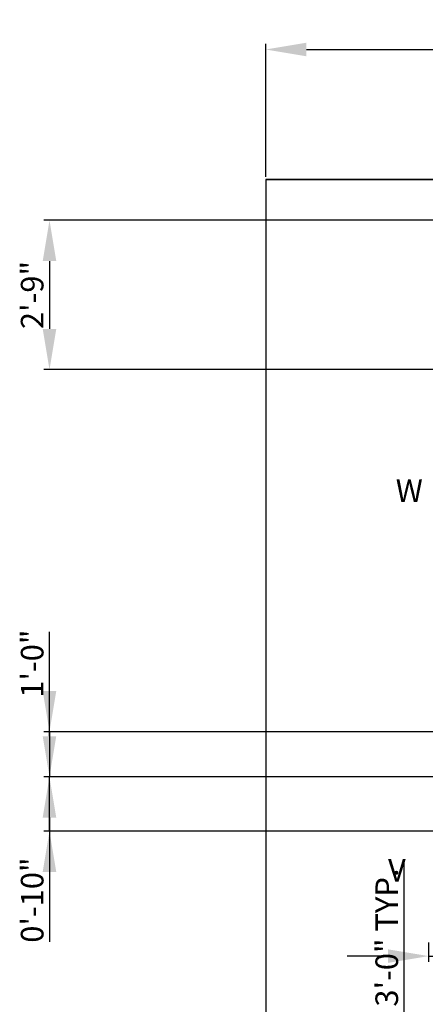
# Model space of a CAD drawing. Units: inches. Extents: x 2265 to 2807, y 1544 to 2401.
# Tile 3 of 9: x 2269 to 2358, y 2073 to 2291. Entities that reach past the tile are written whole.
import ezdxf

# ---------------------------------------------------------------- set-up
doc = ezdxf.new("R2010")
doc.units = ezdxf.units.IN
for name, color, linetype, lineweight in [('A-ANNO-DIMS', 2, 'Continuous', 18), ('A-ANNO-TEXT', 7, 'Continuous', 18), ('A-WALL', 7, 'Continuous', 35), ('C-PROP', 7, 'Continuous', 25)]:
    doc.layers.add(name, color=color, linetype=linetype, lineweight=lineweight)
doc.styles.add('ARIAL', font='times.ttf', dxfattribs={"height": 5})
doc.styles.get("Standard").update_dxf_attribs({"font": 'arial.ttf', "height": 5})
doc.dimstyles.new('ISO-25', dxfattribs={"dimtxt": 5, "dimasz": 9, "dimexe": 1.25, "dimexo": 0.625, "dimtad": 1, "dimlunit": 3, "dimtxsty": 'Standard', "dimcen": 2.5, "dimadec": 0, "dimazin": 0, "dimtfac": 1, "dimtmove": 0, "dimatfit": 3, "dimfxl": 1, "dimarcsym": 0})

# ---------------------------------------------------------------- blocks, each defined once
blk = doc.blocks.new('*D5')
at = {"layer": 'A-ANNO-DIMS', "color": 0, "lineweight": -2, "transparency": 16777216}
for p, q in [((2323.1, 2256.36), (2323.1, 2285.73)), ((2707.1, 2256.36), (2707.1, 2285.73)), ((2332.1, 2284.48), (2698.1, 2284.48))]:
    blk.add_line(p, q, dxfattribs=at)
at = {"layer": 'A-ANNO-DIMS', "color": 0, "lineweight": 100, "transparency": 16777216}
for points in [[(2332.1, 2285.98), (2332.1, 2282.98), (2323.1, 2284.48)], [(2698.1, 2285.98), (2698.1, 2282.98), (2707.1, 2284.48)]]:
    blk.add_solid(points, dxfattribs=at)
at = {"layer": 'Defpoints', "color": 0, "lineweight": 100, "transparency": 16777216}
for p in [(2707.1, 2284.48), (2323.1, 2255.73), (2707.1, 2255.73)]:
    blk.add_point(p, dxfattribs=at)
at = {"layer": 'A-ANNO-DIMS', "color": 0, "transparency": 16777216, "insert": (2515.1, 2287.66), "char_height": 5, "attachment_point": 5}
blk.add_mtext("32'", dxfattribs=at)
blk = doc.blocks.new('*D17')
at = {"layer": 'A-ANNO-DIMS', "color": 0, "lineweight": -2, "transparency": 16777216}
for p, q in [((2353.7, 2031.88), (2353.7, 2105.4)), ((2358.48, 2031.88), (2352.45, 2031.88)), ((2353.7, 2004.88), (2353.7, 2022.88)), ((2358.48, 1995.88), (2352.45, 1995.88))]:
    blk.add_line(p, q, dxfattribs=at)
at = {"layer": 'A-ANNO-DIMS', "color": 0, "lineweight": 100, "transparency": 16777216}
for points in [[(2352.2, 2022.88), (2355.2, 2022.88), (2353.7, 2031.88)], [(2352.2, 2004.88), (2355.2, 2004.88), (2353.7, 1995.88)]]:
    blk.add_solid(points, dxfattribs=at)
at = {"layer": 'Defpoints', "color": 0, "lineweight": 100, "transparency": 16777216}
for p in [(2353.7, 2031.88), (2359.1, 2031.88), (2359.1, 1995.88)]:
    blk.add_point(p, dxfattribs=at)
at = {"layer": 'A-ANNO-DIMS', "color": 0, "transparency": 16777216, "insert": (2350.49, 2073.14), "char_height": 5, "attachment_point": 5, "rotation": 90}
blk.add_mtext('WINDOW 3\'-0" TYP.', dxfattribs=at)
blk = doc.blocks.new('*D21')
at = {"layer": 'A-ANNO-DIMS', "color": 0, "lineweight": -2, "transparency": 16777216}
for p, q in [((2371.7, 2111.73), (2371.7, 2184.98)), ((2368.73, 2111.73), (2372.95, 2111.73)), ((2371.7, 2096.73), (2371.7, 2102.73)), ((2368.73, 2087.73), (2372.95, 2087.73))]:
    blk.add_line(p, q, dxfattribs=at)
at = {"layer": 'A-ANNO-DIMS', "color": 0, "lineweight": 100, "transparency": 16777216}
for points in [[(2370.2, 2102.73), (2373.2, 2102.73), (2371.7, 2111.73)], [(2370.2, 2096.73), (2373.2, 2096.73), (2371.7, 2087.73)]]:
    blk.add_solid(points, dxfattribs=at)
at = {"layer": 'Defpoints', "color": 0, "lineweight": 100, "transparency": 16777216}
for p in [(2368.1, 2111.73), (2371.7, 2111.73), (2368.1, 2087.73)]:
    blk.add_point(p, dxfattribs=at)
at = {"layer": 'A-ANNO-DIMS', "color": 0, "transparency": 16777216, "insert": (2368.49, 2152.86), "char_height": 5, "attachment_point": 5, "rotation": 90}
blk.add_mtext('GLAZING 2\'-0" TYP.', dxfattribs=at)
blk = doc.blocks.new('*D22')
at = {"layer": 'A-ANNO-DIMS', "color": 0, "lineweight": -2, "transparency": 16777216}
for p, q in [((2359.1, 2087.11), (2359.1, 2082.88)), ((2368.1, 2087.11), (2368.1, 2082.88)), ((2350.1, 2084.13), (2341.1, 2084.13)), ((2359.1, 2084.13), (2368.1, 2084.13)), ((2377.1, 2084.13), (2417.83, 2084.13))]:
    blk.add_line(p, q, dxfattribs=at)
at = {"layer": 'A-ANNO-DIMS', "color": 0, "lineweight": 100, "transparency": 16777216}
for points in [[(2350.1, 2085.63), (2350.1, 2082.63), (2359.1, 2084.13)], [(2377.1, 2085.63), (2377.1, 2082.63), (2368.1, 2084.13)]]:
    blk.add_solid(points, dxfattribs=at)
at = {"layer": 'Defpoints', "color": 0, "lineweight": 100, "transparency": 16777216}
for p in [(2359.1, 2087.73), (2368.1, 2087.73), (2368.1, 2084.13)]:
    blk.add_point(p, dxfattribs=at)
at = {"layer": 'A-ANNO-DIMS', "color": 0, "transparency": 16777216, "insert": (2401.96, 2087.31), "char_height": 5, "attachment_point": 5}
blk.add_mtext('0\'-9" TYP.', dxfattribs=at)
blk = doc.blocks.new('*D49')
at = {"layer": 'A-ANNO-DIMS', "color": 0, "lineweight": -2, "transparency": 16777216}
for p, q in [((2275.29, 2132.73), (2275.29, 2155.8)), ((2367.48, 2123.73), (2274.04, 2123.73)), ((2275.29, 2111.73), (2275.29, 2123.73)), ((2367.48, 2111.73), (2274.04, 2111.73)), ((2275.29, 2102.73), (2275.29, 2093.73))]:
    blk.add_line(p, q, dxfattribs=at)
at = {"layer": 'A-ANNO-DIMS', "color": 0, "lineweight": 100, "transparency": 16777216}
for points in [[(2273.79, 2132.73), (2276.79, 2132.73), (2275.29, 2123.73)], [(2273.79, 2102.73), (2276.79, 2102.73), (2275.29, 2111.73)]]:
    blk.add_solid(points, dxfattribs=at)
at = {"layer": 'Defpoints', "color": 0, "lineweight": 100, "transparency": 16777216}
for p in [(2275.29, 2123.73), (2368.1, 2123.73), (2368.1, 2111.73)]:
    blk.add_point(p, dxfattribs=at)
at = {"layer": 'A-ANNO-DIMS', "color": 0, "transparency": 16777216, "insert": (2272.11, 2148.77), "char_height": 5, "attachment_point": 5, "rotation": 90}
blk.add_mtext('1\'-0"', dxfattribs=at)
blk = doc.blocks.new('*D59')
at = {"layer": 'A-ANNO-DIMS', "color": 0, "lineweight": -2, "transparency": 16777216}
for p, q in [((2580.48, 2246.73), (2274.04, 2246.73)), ((2275.29, 2237.73), (2275.29, 2222.73)), ((2580.48, 2213.73), (2274.04, 2213.73))]:
    blk.add_line(p, q, dxfattribs=at)
at = {"layer": 'A-ANNO-DIMS', "color": 0, "lineweight": 100, "transparency": 16777216}
for points in [[(2273.79, 2237.73), (2276.79, 2237.73), (2275.29, 2246.73)], [(2273.79, 2222.73), (2276.79, 2222.73), (2275.29, 2213.73)]]:
    blk.add_solid(points, dxfattribs=at)
at = {"layer": 'Defpoints', "color": 0, "lineweight": 100, "transparency": 16777216}
for p in [(2581.1, 2246.73), (2275.29, 2213.73), (2581.1, 2213.73)]:
    blk.add_point(p, dxfattribs=at)
at = {"layer": 'A-ANNO-DIMS', "color": 0, "transparency": 16777216, "insert": (2272.11, 2230.23), "char_height": 5, "attachment_point": 5, "rotation": 90}
blk.add_mtext('2\'-9"', dxfattribs=at)
blk = doc.blocks.new('*D60')
at = {"layer": 'A-ANNO-DIMS', "color": 0, "lineweight": -2, "transparency": 16777216}
for p, q in [((2275.29, 2142.73), (2275.29, 2151.73)), ((2580.48, 2133.73), (2274.04, 2133.73)), ((2275.29, 2133.73), (2275.29, 2123.73)), ((2580.48, 2123.73), (2274.04, 2123.73)), ((2275.29, 2114.73), (2275.29, 2087.31))]:
    blk.add_line(p, q, dxfattribs=at)
at = {"layer": 'A-ANNO-DIMS', "color": 0, "lineweight": 100, "transparency": 16777216}
for points in [[(2273.79, 2142.73), (2276.79, 2142.73), (2275.29, 2133.73)], [(2273.79, 2114.73), (2276.79, 2114.73), (2275.29, 2123.73)]]:
    blk.add_solid(points, dxfattribs=at)
at = {"layer": 'Defpoints', "color": 0, "lineweight": 100, "transparency": 16777216}
for p in [(2581.1, 2133.73), (2275.29, 2123.73), (2581.1, 2123.73)]:
    blk.add_point(p, dxfattribs=at)
at = {"layer": 'A-ANNO-DIMS', "color": 0, "transparency": 16777216, "insert": (2272.11, 2096.52), "char_height": 5, "attachment_point": 5, "rotation": 90}
blk.add_mtext('0\'-10"', dxfattribs=at)

msp = doc.modelspace()

# ---------------------------------------------------------------- linework, layer by layer
at = {"layer": 'A-WALL'}
msp.add_line((2323.101, 2255.733), (2707.101, 2255.733), dxfattribs=at)
at = {"layer": 'C-PROP'}
msp.add_line((2323.101, 2255.733), (2323.101, 1805.733), dxfattribs=at)

# ---------------------------------------------------------------- texts
at = {"layer": 'A-ANNO-TEXT', "style": 'ARIAL'}
for s, p in [('W', (2351.826, 2184.485)), ('V', (2350.12, 2100.604))]:
    msp.add_text(s, height=5, dxfattribs=at).set_placement(p)

# ---------------------------------------------------------------- dimensions: what is measured, and where the dimension line sits
at = {"layer": 'A-ANNO-DIMS'}
dim = msp.add_linear_dim(base=(2707.101, 2284.48), p1=(2323.101, 2255.733), p2=(2707.101, 2255.733), dimstyle='ISO-25', override={"dimclrd": 0, "dimclre": 0, "dimclrt": 0}, dxfattribs=at)
dim.commit()
dim.dimension.update_dxf_attribs({"geometry": '*D5', "text_midpoint": (2515.101, 2287.659)})
for base, p1, p2, picture, middle in [((2275.289, 2213.733), (2581.101, 2246.733), (2581.101, 2213.733), '*D59', (2272.111, 2230.233)), ((2275.289, 2123.733), (2368.101, 2111.733), (2368.101, 2123.733), '*D49', (2272.111, 2148.769)), ((2275.289, 2123.733), (2581.101, 2133.733), (2581.101, 2123.733), '*D60', (2272.111, 2096.52))]:
    dim = msp.add_linear_dim(base=base, p1=p1, p2=p2, angle=90, dimstyle='ISO-25', override={"dimdec": 1, "dimlfac": 1, "dimrnd": 0, "dimzin": 1, "dimdsep": 46, "dimlunit": 4, "dimfrac": 2}, dxfattribs=at)
    dim.commit()
    dim.dimension.update_dxf_attribs({"geometry": picture, "text_midpoint": middle})
for base, p1, p2, text, picture, middle in [((2371.701, 2111.733), (2368.101, 2087.733), (2368.101, 2111.733), 'GLAZING <> TYP.', '*D21', (2368.491, 2152.857)), ((2353.701, 2031.884), (2359.101, 1995.884), (2359.101, 2031.884), 'WINDOW <> TYP.', '*D17', (2350.488, 2073.144))]:
    dim = msp.add_linear_dim(base=base, p1=p1, p2=p2, angle=90, text=text, dimstyle='ISO-25', override={"dimdec": 1, "dimlfac": 1, "dimrnd": 0, "dimzin": 1, "dimdsep": 46, "dimlunit": 4, "dimfrac": 2}, dxfattribs=at)
    dim.commit()
    dim.dimension.update_dxf_attribs({"geometry": picture, "text_midpoint": middle})
dim = msp.add_linear_dim(base=(2368.101, 2084.133), p1=(2359.101, 2087.733), p2=(2368.101, 2087.733), text='<> TYP.', dimstyle='ISO-25', override={"dimdec": 1, "dimlfac": 1, "dimrnd": 0, "dimzin": 1, "dimdsep": 46, "dimlunit": 4, "dimfrac": 2}, dxfattribs=at)
dim.commit()
dim.dimension.update_dxf_attribs({"geometry": '*D22', "text_midpoint": (2401.965, 2087.311)})

doc.saveas('drawing.dxf')
